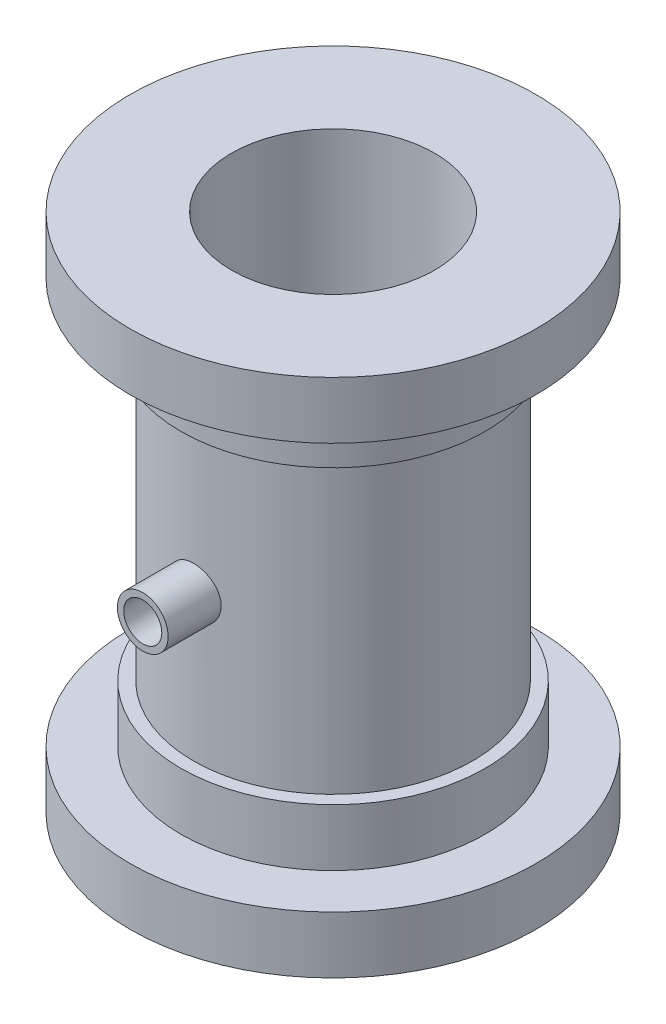
ISO-10303-21;
HEADER;
FILE_DESCRIPTION(('STEP AP214'),'2;1');
FILE_NAME('part.step','',(''),(''),'','','');
FILE_SCHEMA(('AUTOMOTIVE_DESIGN { 1 0 10303 214 1 1 1 1 }'));
ENDSEC;
DATA;
#1=APPLICATION_CONTEXT('core data for automotive mechanical design processes');
#2=APPLICATION_PROTOCOL_DEFINITION('international standard','automotive_design',2000,#1);
#3=PRODUCT_CONTEXT('',#1,'mechanical');
#4=PRODUCT('Part','Part','',(#3));
#5=PRODUCT_RELATED_PRODUCT_CATEGORY('part','',(#4));
#6=PRODUCT_DEFINITION_FORMATION('','',#4);
#7=PRODUCT_DEFINITION_CONTEXT('part definition',#1,'design');
#8=PRODUCT_DEFINITION('design','',#6,#7);
#9=PRODUCT_DEFINITION_SHAPE('','',#8);
#10=(LENGTH_UNIT() NAMED_UNIT(*) SI_UNIT(.MILLI.,.METRE.));
#11=(NAMED_UNIT(*) PLANE_ANGLE_UNIT() SI_UNIT($,.RADIAN.));
#12=(NAMED_UNIT(*) SI_UNIT($,.STERADIAN.) SOLID_ANGLE_UNIT());
#13=UNCERTAINTY_MEASURE_WITH_UNIT(LENGTH_MEASURE(1.E-05),#10,'distance_accuracy_value','');
#14=(GEOMETRIC_REPRESENTATION_CONTEXT(3) GLOBAL_UNCERTAINTY_ASSIGNED_CONTEXT((#13)) GLOBAL_UNIT_ASSIGNED_CONTEXT((#10,
#11,#12)) REPRESENTATION_CONTEXT('',''));
#15=CARTESIAN_POINT('',(0.,0.,0.));
#16=DIRECTION('',(0.,0.,1.));
#17=DIRECTION('',(1.,0.,0.));
#18=AXIS2_PLACEMENT_3D('',#15,#16,#17);
#19=CARTESIAN_POINT('',(0.,206.829787614374,0.));
#20=DIRECTION('',(0.,1.,0.));
#21=DIRECTION('',(0.,0.,1.));
#22=AXIS2_PLACEMENT_3D('',#19,#20,#21);
#23=CYLINDRICAL_SURFACE('',#22,16.);
#24=CARTESIAN_POINT('',(2.99999999999999,41.,-15.7162336455017));
#25=CARTESIAN_POINT('',(2.99999359766588,40.8330855839748,-15.7162368759014));
#26=CARTESIAN_POINT('',(2.98602252697897,40.6660881035627,-15.7189215952138));
#27=CARTESIAN_POINT('',(2.93054506503583,40.3368020768367,-15.7293570202788));
#28=CARTESIAN_POINT('',(2.88901531536946,40.1745176471452,-15.7371120234618));
#29=CARTESIAN_POINT('',(2.77974071235581,39.8594698572581,-15.7567795292999));
#30=CARTESIAN_POINT('',(2.71202027908749,39.7066977813854,-15.7686881581205));
#31=CARTESIAN_POINT('',(2.55235131520729,39.4146928814264,-15.7953165264186));
#32=CARTESIAN_POINT('',(2.46040467518385,39.2754590019934,-15.8100360465123));
#33=CARTESIAN_POINT('',(2.25367357885245,39.0127396016017,-15.840832296779));
#34=CARTESIAN_POINT('',(2.13864585866183,38.8894470330565,-15.8569223325136));
#35=CARTESIAN_POINT('',(1.8895435576071,38.6637912208009,-15.8885291532806));
#36=CARTESIAN_POINT('',(1.75546772724988,38.5614293511504,-15.904045900623));
#37=CARTESIAN_POINT('',(1.47080778914032,38.379801246799,-15.9329003565681));
#38=CARTESIAN_POINT('',(1.32010568006772,38.3007169329612,-15.9462205610472));
#39=CARTESIAN_POINT('',(1.00726256650152,38.1690609154529,-15.9690321726586));
#40=CARTESIAN_POINT('',(0.845122503719006,38.1164870320196,-15.9785238945667));
#41=CARTESIAN_POINT('',(0.516005492374828,38.0399409027777,-15.9925151024756));
#42=CARTESIAN_POINT('',(0.349106646489711,38.0156433881546,-15.9970713195265));
#43=CARTESIAN_POINT('',(0.0135433520707638,37.9953262245992,-16.0008736923119));
#44=CARTESIAN_POINT('',(-0.155120944895342,37.9993041677219,-16.0001203002139));
#45=CARTESIAN_POINT('',(-0.487196715798794,38.0351755422943,-15.9934326752648));
#46=CARTESIAN_POINT('',(-0.650647520902939,38.06671873886,-15.9875634449443));
#47=CARTESIAN_POINT('',(-0.969894331430951,38.1562712987905,-15.9713765266712));
#48=CARTESIAN_POINT('',(-1.12569005765308,38.2142816266916,-15.9610586765993));
#49=CARTESIAN_POINT('',(-1.42622013150304,38.3554554621166,-15.9370252059468));
#50=CARTESIAN_POINT('',(-1.57088714367706,38.438758975825,-15.9232907518165));
#51=CARTESIAN_POINT('',(-1.84431995442927,38.6280513381543,-15.893942950857));
#52=CARTESIAN_POINT('',(-1.97308413382157,38.7340424937752,-15.8783294130233));
#53=CARTESIAN_POINT('',(-2.21313123793807,38.9676314059671,-15.8466702736113));
#54=CARTESIAN_POINT('',(-2.32411581514081,39.0955355678042,-15.8306217180324));
#55=CARTESIAN_POINT('',(-2.5231034370252,39.3682990625573,-15.8001301784924));
#56=CARTESIAN_POINT('',(-2.61110614542363,39.5131586435293,-15.785687218027));
#57=CARTESIAN_POINT('',(-2.76171704448954,39.8161165414053,-15.7600378661424));
#58=CARTESIAN_POINT('',(-2.82428187290842,39.9742369143813,-15.7488370106052));
#59=CARTESIAN_POINT('',(-2.92187313950111,40.2990023682464,-15.7310248479338));
#60=CARTESIAN_POINT('',(-2.95690269802215,40.4656464809296,-15.7244130207724));
#61=CARTESIAN_POINT('',(-2.99799345299477,40.8000386577118,-15.7166304060201));
#62=CARTESIAN_POINT('',(-3.00448328571716,40.967732231131,-15.7153791163227));
#63=CARTESIAN_POINT('',(-2.98945937763448,41.3018069101743,-15.7182438284168));
#64=CARTESIAN_POINT('',(-2.96794702172865,41.4681880802962,-15.7223595647722));
#65=CARTESIAN_POINT('',(-2.89789736391764,41.7935058061088,-15.7354196012641));
#66=CARTESIAN_POINT('',(-2.84958477167978,41.9524925052498,-15.7443237338176));
#67=CARTESIAN_POINT('',(-2.72754448758118,42.2601143794603,-15.7659226831324));
#68=CARTESIAN_POINT('',(-2.65381492257589,42.4087487906307,-15.7786177792656));
#69=CARTESIAN_POINT('',(-2.48204706239319,42.6933352380863,-15.8065515572737));
#70=CARTESIAN_POINT('',(-2.38373799279241,42.8291210757322,-15.8218179085063));
#71=CARTESIAN_POINT('',(-2.16596688688492,43.0824240804287,-15.853096227362));
#72=CARTESIAN_POINT('',(-2.04650294866166,43.1999396031115,-15.8691082619299));
#73=CARTESIAN_POINT('',(-1.78789883574076,43.4149675270682,-15.9003324801189));
#74=CARTESIAN_POINT('',(-1.64851706819177,43.5121916532119,-15.9155311166661));
#75=CARTESIAN_POINT('',(-1.35514904608027,43.6818424123553,-15.943188096207));
#76=CARTESIAN_POINT('',(-1.20116335407705,43.75427000005,-15.9556465446945));
#77=CARTESIAN_POINT('',(-0.883755083157361,43.8718401957282,-15.9763611599169));
#78=CARTESIAN_POINT('',(-0.72038642615797,43.9171243751228,-15.9846390946028));
#79=CARTESIAN_POINT('',(-0.388192454763134,43.9795740965798,-15.9961528416749));
#80=CARTESIAN_POINT('',(-0.219367716431691,43.9967425973254,-15.9993891845988));
#81=CARTESIAN_POINT('',(0.116181520501017,44.0023706030369,-16.0004445503086));
#82=CARTESIAN_POINT('',(0.282898614132518,43.9912655062591,-15.9983457325));
#83=CARTESIAN_POINT('',(0.612046738558423,43.9416151444631,-15.9891373322347));
#84=CARTESIAN_POINT('',(0.774477810427464,43.9030701425114,-15.9820277978157));
#85=CARTESIAN_POINT('',(1.09021295119089,43.7998175852327,-15.9635967595586));
#86=CARTESIAN_POINT('',(1.24353263863614,43.7351563742386,-15.9522827196228));
#87=CARTESIAN_POINT('',(1.5372112626337,43.581559092689,-15.9266674413841));
#88=CARTESIAN_POINT('',(1.67756933000769,43.4926213957845,-15.912366002962));
#89=CARTESIAN_POINT('',(1.94351005555884,43.2914970911175,-15.882095597166));
#90=CARTESIAN_POINT('',(2.06885247077666,43.1789959322848,-15.8661056917023));
#91=CARTESIAN_POINT('',(2.29903072131409,42.9345908750064,-15.8343926708998));
#92=CARTESIAN_POINT('',(2.403861726512,42.8026824192219,-15.8186696191953));
#93=CARTESIAN_POINT('',(2.59095267889405,42.5217470906199,-15.7891115480538));
#94=CARTESIAN_POINT('',(2.67299481058046,42.3725731207714,-15.7752953438736));
#95=CARTESIAN_POINT('',(2.8107226484115,42.0623484201479,-15.7513416912985));
#96=CARTESIAN_POINT('',(2.86643323276462,41.9013090668493,-15.7412007725928));
#97=CARTESIAN_POINT('',(2.93859453193229,41.6164954238523,-15.7278603261271));
#98=CARTESIAN_POINT('',(2.96158211479938,41.4943885524718,-15.7235262144357));
#99=CARTESIAN_POINT('',(2.99228702152191,41.2482030631637,-15.7177117118331));
#100=CARTESIAN_POINT('',(3.00000476104181,41.1241244990007,-15.7162312432422));
#101=CARTESIAN_POINT('',(2.99999999999999,41.,-15.7162336455017));
#102=B_SPLINE_CURVE_WITH_KNOTS('',3,(#24,#25,#26,#27,#28,#29,#30,#31,#32,#33,#34,#35,#36,#37,
#38,#39,#40,#41,#42,#43,#44,#45,#46,#47,#48,#49,#50,#51,#52,#53,#54,#55,#56,#57,#58,#59,#60,#61,
#62,#63,#64,#65,#66,#67,#68,#69,#70,#71,#72,#73,#74,#75,#76,#77,#78,#79,#80,#81,#82,#83,#84,#85,
#86,#87,#88,#89,#90,#91,#92,#93,#94,#95,#96,#97,#98,#99,#100,#101),.UNSPECIFIED.,.T.,.F.,(4,2,2,
2,2,2,2,2,2,2,2,2,2,2,2,2,2,2,2,2,2,2,2,2,2,2,2,2,2,2,2,2,2,2,2,2,2,2,4),(0.,0.500289011586363,
1.00100260476078,1.50125045595686,2.00145927987815,2.50724671397381,3.01306734138628,
3.52274208696094,4.03237491879279,4.53608550920521,5.03975320401295,5.53711301197448,
6.03449094656847,6.53467383968437,7.03490761823569,7.54281229528126,8.05072440384797,
8.5594987223653,9.06821537732973,9.56926497174148,10.0702897867743,10.5671758463073,
11.0640985324863,11.5667572530828,12.0694611878935,12.5788825099174,13.0882842164341,
13.5950053883736,14.1016732333466,14.6005860114027,15.0994940064433,15.5975205306071,
16.0955804271421,16.6007692801748,17.1060769546152,17.6160600363781,18.1255603150175,
18.4976061505794,18.8696418584436),.UNSPECIFIED.);
#103=CARTESIAN_POINT('',(2.99999999999999,41.,-15.7162336455017));
#104=VERTEX_POINT('',#103);
#105=EDGE_CURVE('E41',#104,#104,#102,.T.);
#106=ORIENTED_EDGE('',*,*,#105,.T.);
#107=EDGE_LOOP('',(#106));
#108=FACE_BOUND('',#107,.T.);
#109=CARTESIAN_POINT('',(0.,0.,0.));
#110=DIRECTION('',(0.,1.,0.));
#111=DIRECTION('',(0.,0.,1.));
#112=AXIS2_PLACEMENT_3D('',#109,#110,#111);
#113=CIRCLE('',#112,16.);
#114=CARTESIAN_POINT('',(0.,0.,16.));
#115=VERTEX_POINT('',#114);
#116=EDGE_CURVE('E52',#115,#115,#113,.T.);
#117=ORIENTED_EDGE('',*,*,#116,.F.);
#118=EDGE_LOOP('',(#117));
#119=FACE_BOUND('',#118,.T.);
#120=CARTESIAN_POINT('',(0.,82.,0.));
#121=DIRECTION('',(0.,1.,0.));
#122=DIRECTION('',(0.,0.,1.));
#123=AXIS2_PLACEMENT_3D('',#120,#121,#122);
#124=CIRCLE('',#123,16.);
#125=CARTESIAN_POINT('',(0.,82.,16.));
#126=VERTEX_POINT('',#125);
#127=EDGE_CURVE('E47',#126,#126,#124,.T.);
#128=ORIENTED_EDGE('',*,*,#127,.T.);
#129=EDGE_LOOP('',(#128));
#130=FACE_BOUND('',#129,.T.);
#131=CARTESIAN_POINT('',(2.99999999999999,41.,15.7162336455017));
#132=CARTESIAN_POINT('',(2.99999359766588,40.8330855839748,15.7162368759014));
#133=CARTESIAN_POINT('',(2.98602252697897,40.6660881035627,15.7189215952138));
#134=CARTESIAN_POINT('',(2.93054506503583,40.3368020768367,15.7293570202788));
#135=CARTESIAN_POINT('',(2.88901531536946,40.1745176471452,15.7371120234618));
#136=CARTESIAN_POINT('',(2.77974071235581,39.8594698572581,15.7567795292999));
#137=CARTESIAN_POINT('',(2.71202027908749,39.7066977813854,15.7686881581205));
#138=CARTESIAN_POINT('',(2.55235131520729,39.4146928814264,15.7953165264186));
#139=CARTESIAN_POINT('',(2.46040467518385,39.2754590019934,15.8100360465123));
#140=CARTESIAN_POINT('',(2.25367357885245,39.0127396016017,15.840832296779));
#141=CARTESIAN_POINT('',(2.13864585866183,38.8894470330565,15.8569223325136));
#142=CARTESIAN_POINT('',(1.8895435576071,38.6637912208009,15.8885291532806));
#143=CARTESIAN_POINT('',(1.75546772724988,38.5614293511504,15.904045900623));
#144=CARTESIAN_POINT('',(1.47080778914032,38.379801246799,15.9329003565681));
#145=CARTESIAN_POINT('',(1.32010568006772,38.3007169329612,15.9462205610472));
#146=CARTESIAN_POINT('',(1.00726256650152,38.1690609154529,15.9690321726586));
#147=CARTESIAN_POINT('',(0.845122503719006,38.1164870320196,15.9785238945667));
#148=CARTESIAN_POINT('',(0.516005492374828,38.0399409027777,15.9925151024756));
#149=CARTESIAN_POINT('',(0.349106646489711,38.0156433881546,15.9970713195265));
#150=CARTESIAN_POINT('',(0.0135433520707638,37.9953262245992,16.0008736923119));
#151=CARTESIAN_POINT('',(-0.155120944895342,37.9993041677219,16.0001203002139));
#152=CARTESIAN_POINT('',(-0.487196715798794,38.0351755422943,15.9934326752648));
#153=CARTESIAN_POINT('',(-0.650647520902939,38.06671873886,15.9875634449443));
#154=CARTESIAN_POINT('',(-0.969894331430951,38.1562712987905,15.9713765266712));
#155=CARTESIAN_POINT('',(-1.12569005765308,38.2142816266916,15.9610586765993));
#156=CARTESIAN_POINT('',(-1.42622013150304,38.3554554621166,15.9370252059468));
#157=CARTESIAN_POINT('',(-1.57088714367706,38.438758975825,15.9232907518165));
#158=CARTESIAN_POINT('',(-1.84431995442927,38.6280513381543,15.893942950857));
#159=CARTESIAN_POINT('',(-1.97308413382157,38.7340424937752,15.8783294130233));
#160=CARTESIAN_POINT('',(-2.21313123793807,38.9676314059671,15.8466702736113));
#161=CARTESIAN_POINT('',(-2.32411581514081,39.0955355678042,15.8306217180324));
#162=CARTESIAN_POINT('',(-2.5231034370252,39.3682990625573,15.8001301784924));
#163=CARTESIAN_POINT('',(-2.61110614542363,39.5131586435293,15.785687218027));
#164=CARTESIAN_POINT('',(-2.76171704448954,39.8161165414053,15.7600378661424));
#165=CARTESIAN_POINT('',(-2.82428187290842,39.9742369143813,15.7488370106052));
#166=CARTESIAN_POINT('',(-2.92187313950111,40.2990023682464,15.7310248479338));
#167=CARTESIAN_POINT('',(-2.95690269802215,40.4656464809296,15.7244130207724));
#168=CARTESIAN_POINT('',(-2.99799345299477,40.8000386577118,15.7166304060201));
#169=CARTESIAN_POINT('',(-3.00448328571716,40.967732231131,15.7153791163227));
#170=CARTESIAN_POINT('',(-2.98945937763448,41.3018069101743,15.7182438284168));
#171=CARTESIAN_POINT('',(-2.96794702172865,41.4681880802962,15.7223595647722));
#172=CARTESIAN_POINT('',(-2.89789736391764,41.7935058061088,15.7354196012641));
#173=CARTESIAN_POINT('',(-2.84958477167978,41.9524925052498,15.7443237338176));
#174=CARTESIAN_POINT('',(-2.72754448758118,42.2601143794603,15.7659226831324));
#175=CARTESIAN_POINT('',(-2.65381492257589,42.4087487906307,15.7786177792656));
#176=CARTESIAN_POINT('',(-2.48204706239319,42.6933352380863,15.8065515572737));
#177=CARTESIAN_POINT('',(-2.38373799279241,42.8291210757322,15.8218179085063));
#178=CARTESIAN_POINT('',(-2.16596688688492,43.0824240804287,15.853096227362));
#179=CARTESIAN_POINT('',(-2.04650294866166,43.1999396031115,15.8691082619299));
#180=CARTESIAN_POINT('',(-1.78789883574076,43.4149675270682,15.9003324801189));
#181=CARTESIAN_POINT('',(-1.64851706819177,43.5121916532119,15.9155311166661));
#182=CARTESIAN_POINT('',(-1.35514904608027,43.6818424123553,15.943188096207));
#183=CARTESIAN_POINT('',(-1.20116335407705,43.75427000005,15.9556465446945));
#184=CARTESIAN_POINT('',(-0.883755083157361,43.8718401957282,15.9763611599169));
#185=CARTESIAN_POINT('',(-0.72038642615797,43.9171243751228,15.9846390946028));
#186=CARTESIAN_POINT('',(-0.388192454763134,43.9795740965798,15.9961528416749));
#187=CARTESIAN_POINT('',(-0.219367716431691,43.9967425973254,15.9993891845988));
#188=CARTESIAN_POINT('',(0.116181520501017,44.0023706030369,16.0004445503086));
#189=CARTESIAN_POINT('',(0.282898614132518,43.9912655062591,15.9983457325));
#190=CARTESIAN_POINT('',(0.612046738558423,43.9416151444631,15.9891373322347));
#191=CARTESIAN_POINT('',(0.774477810427464,43.9030701425114,15.9820277978157));
#192=CARTESIAN_POINT('',(1.09021295119089,43.7998175852327,15.9635967595586));
#193=CARTESIAN_POINT('',(1.24353263863614,43.7351563742386,15.9522827196228));
#194=CARTESIAN_POINT('',(1.5372112626337,43.581559092689,15.9266674413841));
#195=CARTESIAN_POINT('',(1.67756933000769,43.4926213957845,15.912366002962));
#196=CARTESIAN_POINT('',(1.94351005555884,43.2914970911175,15.882095597166));
#197=CARTESIAN_POINT('',(2.06885247077666,43.1789959322848,15.8661056917023));
#198=CARTESIAN_POINT('',(2.29903072131409,42.9345908750064,15.8343926708998));
#199=CARTESIAN_POINT('',(2.403861726512,42.8026824192219,15.8186696191953));
#200=CARTESIAN_POINT('',(2.59095267889405,42.5217470906199,15.7891115480538));
#201=CARTESIAN_POINT('',(2.67299481058046,42.3725731207714,15.7752953438736));
#202=CARTESIAN_POINT('',(2.8107226484115,42.0623484201479,15.7513416912985));
#203=CARTESIAN_POINT('',(2.86643323276462,41.9013090668493,15.7412007725928));
#204=CARTESIAN_POINT('',(2.93859453193229,41.6164954238523,15.7278603261271));
#205=CARTESIAN_POINT('',(2.96158211479938,41.4943885524718,15.7235262144357));
#206=CARTESIAN_POINT('',(2.99228702152191,41.2482030631637,15.7177117118331));
#207=CARTESIAN_POINT('',(3.00000476104181,41.1241244990007,15.7162312432422));
#208=CARTESIAN_POINT('',(2.99999999999999,41.,15.7162336455017));
#209=B_SPLINE_CURVE_WITH_KNOTS('',3,(#131,#132,#133,#134,#135,#136,#137,#138,#139,#140,#141,
#142,#143,#144,#145,#146,#147,#148,#149,#150,#151,#152,#153,#154,#155,#156,#157,#158,#159,#160,
#161,#162,#163,#164,#165,#166,#167,#168,#169,#170,#171,#172,#173,#174,#175,#176,#177,#178,#179,
#180,#181,#182,#183,#184,#185,#186,#187,#188,#189,#190,#191,#192,#193,#194,#195,#196,#197,#198,
#199,#200,#201,#202,#203,#204,#205,#206,#207,#208),.UNSPECIFIED.,.T.,.F.,(4,2,2,2,2,2,2,2,2,2,2,
2,2,2,2,2,2,2,2,2,2,2,2,2,2,2,2,2,2,2,2,2,2,2,2,2,2,2,4),(0.,0.500289011586363,1.00100260476078,
1.50125045595686,2.00145927987815,2.50724671397381,3.01306734138628,3.52274208696094,
4.03237491879279,4.53608550920521,5.03975320401295,5.53711301197448,6.03449094656847,
6.53467383968437,7.03490761823569,7.54281229528126,8.05072440384797,8.5594987223653,
9.06821537732973,9.56926497174148,10.0702897867743,10.5671758463073,11.0640985324863,
11.5667572530828,12.0694611878935,12.5788825099174,13.0882842164341,13.5950053883736,
14.1016732333466,14.6005860114027,15.0994940064433,15.5975205306071,16.0955804271421,
16.6007692801748,17.1060769546152,17.6160600363781,18.1255603150175,18.4976061505794,
18.8696418584436),.UNSPECIFIED.);
#210=CARTESIAN_POINT('',(2.99999999999999,41.,15.7162336455017));
#211=VERTEX_POINT('',#210);
#212=EDGE_CURVE('E149',#211,#211,#209,.T.);
#213=ORIENTED_EDGE('',*,*,#212,.F.);
#214=EDGE_LOOP('',(#213));
#215=FACE_BOUND('',#214,.T.);
#216=ADVANCED_FACE('F40',(#108,#119,#130,#215),#23,.F.);
#217=CARTESIAN_POINT('',(0.,206.829787614374,0.));
#218=DIRECTION('',(0.,1.,0.));
#219=DIRECTION('',(0.,0.,1.));
#220=AXIS2_PLACEMENT_3D('',#217,#218,#219);
#221=CYLINDRICAL_SURFACE('',#220,22.);
#222=CARTESIAN_POINT('',(2.99999999999999,41.,-21.7944947177034));
#223=CARTESIAN_POINT('',(2.99999295397828,41.1676686557939,-21.7944973125222));
#224=CARTESIAN_POINT('',(2.98589613516891,41.335438885572,-21.7964504822141));
#225=CARTESIAN_POINT('',(2.92988930626151,41.6663009494034,-21.8040481680046));
#226=CARTESIAN_POINT('',(2.88795106929476,41.8293878600565,-21.8096964302678));
#227=CARTESIAN_POINT('',(2.7775288562679,42.1460455710164,-21.8240329226108));
#228=CARTESIAN_POINT('',(2.70906391400625,42.2996231031868,-21.8327189725423));
#229=CARTESIAN_POINT('',(2.54757436301585,42.593083937498,-21.8521497354893));
#230=CARTESIAN_POINT('',(2.4545535979434,42.7329693781315,-21.8628941262462));
#231=CARTESIAN_POINT('',(2.24593261550095,42.9960291899694,-21.8853107439761));
#232=CARTESIAN_POINT('',(2.13020174404837,43.1190995206715,-21.8969880962733));
#233=CARTESIAN_POINT('',(1.87972745186893,43.3441356113716,-21.9199089625179));
#234=CARTESIAN_POINT('',(1.74498304377951,43.446100274685,-21.9311524538967));
#235=CARTESIAN_POINT('',(1.45964673364284,43.6264088097933,-21.9519917823356));
#236=CARTESIAN_POINT('',(1.30899431491146,43.7046577531438,-21.9615809332171));
#237=CARTESIAN_POINT('',(0.996533559622191,43.8347051362175,-21.9779746087792));
#238=CARTESIAN_POINT('',(0.834725713012592,43.8865047367613,-21.9847792556648));
#239=CARTESIAN_POINT('',(0.505615027627403,43.9618700639319,-21.9948010960819));
#240=CARTESIAN_POINT('',(0.338352625202418,43.9856093917029,-21.9980403391051));
#241=CARTESIAN_POINT('',(0.00218901989865064,44.0047187619281,-22.0006418160325));
#242=CARTESIAN_POINT('',(-0.166712106612742,44.0000901200993,-22.0000042297454));
#243=CARTESIAN_POINT('',(-0.500176134095491,43.9627331448272,-21.9949416293269));
#244=CARTESIAN_POINT('',(-0.664760389901238,43.9301915409683,-21.9905417842193));
#245=CARTESIAN_POINT('',(-0.986109968659578,43.8382247979685,-21.9784771616625));
#246=CARTESIAN_POINT('',(-1.1428751195119,43.7787990673916,-21.9708123123852));
#247=CARTESIAN_POINT('',(-1.44470900216683,43.6345555950203,-21.9530355245634));
#248=CARTESIAN_POINT('',(-1.58973910165001,43.5496579984127,-21.9429159096715));
#249=CARTESIAN_POINT('',(-1.86356465940336,43.356938901094,-21.9213599095811));
#250=CARTESIAN_POINT('',(-1.99235923191068,43.2491161505149,-21.9099234526045));
#251=CARTESIAN_POINT('',(-2.2311563912285,43.0125639881593,-21.8869019715346));
#252=CARTESIAN_POINT('',(-2.34099765683571,42.883671704982,-21.8753164955576));
#253=CARTESIAN_POINT('',(-2.53751386076588,42.6091960813263,-21.8533940433535));
#254=CARTESIAN_POINT('',(-2.62418869928228,42.4636126689425,-21.8430570725053));
#255=CARTESIAN_POINT('',(-2.77192629130126,42.159733098398,-21.8248023099056));
#256=CARTESIAN_POINT('',(-2.83297454471216,42.0014298032314,-21.816885888441));
#257=CARTESIAN_POINT('',(-2.92757469616753,41.6766859388551,-21.8043941534575));
#258=CARTESIAN_POINT('',(-2.96112818173422,41.5102458400451,-21.7998186470391));
#259=CARTESIAN_POINT('',(-2.99956941672118,41.1753823129862,-21.7945626889125));
#260=CARTESIAN_POINT('',(-3.00468490854896,41.006985496761,-21.7938512929769));
#261=CARTESIAN_POINT('',(-2.98670732293098,40.6717371641337,-21.7963221316711));
#262=CARTESIAN_POINT('',(-2.96361496443093,40.5048856084559,-21.7995042670648));
#263=CARTESIAN_POINT('',(-2.89006955453773,40.1781565348422,-21.8093753071634));
#264=CARTESIAN_POINT('',(-2.83972815512374,40.0182534145076,-21.8160498979624));
#265=CARTESIAN_POINT('',(-2.71322912313732,39.7091565507405,-21.8321421092609));
#266=CARTESIAN_POINT('',(-2.63707042220061,39.5599632508084,-21.8415598432741));
#267=CARTESIAN_POINT('',(-2.46054424209314,39.2754947875546,-21.8621508077798));
#268=CARTESIAN_POINT('',(-2.36002824545062,39.1403125677473,-21.8733346554527));
#269=CARTESIAN_POINT('',(-2.13784918546697,38.8886549951314,-21.8961649833416));
#270=CARTESIAN_POINT('',(-2.01618513932771,38.7721805121983,-21.9078114850387));
#271=CARTESIAN_POINT('',(-1.7541651749027,38.5604369463813,-21.9303506440045));
#272=CARTESIAN_POINT('',(-1.61368731048534,38.4653180710751,-21.9412376115705));
#273=CARTESIAN_POINT('',(-1.31861563564172,38.3000282219224,-21.9609445601932));
#274=CARTESIAN_POINT('',(-1.16402215510119,38.229856665238,-21.9697645895377));
#275=CARTESIAN_POINT('',(-0.845593617063874,38.116697948143,-21.9843187797623));
#276=CARTESIAN_POINT('',(-0.681789143548591,38.0736260127072,-21.9900625555325));
#277=CARTESIAN_POINT('',(-0.349189125620999,38.0156139846478,-21.9978571930975));
#278=CARTESIAN_POINT('',(-0.18039385182202,38.0006723695607,-21.9999082547485));
#279=CARTESIAN_POINT('',(0.155933944793781,37.9993773344575,-22.0000849669784));
#280=CARTESIAN_POINT('',(0.323465608546994,38.0127930862346,-21.9982423123403));
#281=CARTESIAN_POINT('',(0.65386852750444,38.0673405312772,-21.9909020074537));
#282=CARTESIAN_POINT('',(0.816739790572315,38.1084721777741,-21.9854043633727));
#283=CARTESIAN_POINT('',(1.13315387765858,38.2172071855912,-21.9713688879314));
#284=CARTESIAN_POINT('',(1.28670131426866,38.2847973323295,-21.9628325744139));
#285=CARTESIAN_POINT('',(1.58031159285156,38.4445066044813,-21.9436616719154));
#286=CARTESIAN_POINT('',(1.72037415250691,38.5366262432889,-21.9330270390184));
#287=CARTESIAN_POINT('',(1.98421472860386,38.7436255734436,-21.9107413064255));
#288=CARTESIAN_POINT('',(2.10785776937318,38.8586765359164,-21.899082951343));
#289=CARTESIAN_POINT('',(2.33416948478684,39.1079137559864,-21.8761200052605));
#290=CARTESIAN_POINT('',(2.43683320845294,39.2421045177904,-21.864815498298));
#291=CARTESIAN_POINT('',(2.61868613380123,39.5265296933573,-21.8437846234674));
#292=CARTESIAN_POINT('',(2.69776514213642,39.6768350915978,-21.8340657568726));
#293=CARTESIAN_POINT('',(2.82944291998179,39.9886475846397,-21.817394367016));
#294=CARTESIAN_POINT('',(2.8820699216208,40.1501425264417,-21.8104388960614));
#295=CARTESIAN_POINT('',(2.94703203226376,40.427022796486,-21.8017355288375));
#296=CARTESIAN_POINT('',(2.96686567785598,40.5406764223968,-21.7990341203125));
#297=CARTESIAN_POINT('',(2.99335201931174,40.7695373771214,-21.7954128315745));
#298=CARTESIAN_POINT('',(3.00000484343007,40.8847446908062,-21.7944929340268));
#299=CARTESIAN_POINT('',(2.99999999999999,41.,-21.7944947177034));
#300=B_SPLINE_CURVE_WITH_KNOTS('',3,(#222,#223,#224,#225,#226,#227,#228,#229,#230,#231,#232,
#233,#234,#235,#236,#237,#238,#239,#240,#241,#242,#243,#244,#245,#246,#247,#248,#249,#250,#251,
#252,#253,#254,#255,#256,#257,#258,#259,#260,#261,#262,#263,#264,#265,#266,#267,#268,#269,#270,
#271,#272,#273,#274,#275,#276,#277,#278,#279,#280,#281,#282,#283,#284,#285,#286,#287,#288,#289,
#290,#291,#292,#293,#294,#295,#296,#297,#298,#299),.UNSPECIFIED.,.T.,.F.,(4,2,2,2,2,2,2,2,2,2,2,
2,2,2,2,2,2,2,2,2,2,2,2,2,2,2,2,2,2,2,2,2,2,2,2,2,2,2,4),(0.,0.502584827322537,1.00567997726411,
1.50841480614355,2.01107098991681,2.51670860353079,3.02237248429927,3.53003447052539,
4.03767417433727,4.54215653413512,5.04661549603349,5.54772586150295,6.04884725166252,
6.55155638132179,7.05429292546102,7.56111742626898,8.06794411056384,8.57505718337531,
9.0821409738876,9.585157927571,10.0881620609109,10.5891205844915,11.0900998411272,
11.5942142584275,12.0983521093422,12.6059319233779,13.1134998781726,13.6194720220333,
14.125416780985,14.627259029653,15.1291004314968,15.6306915099823,16.1322930874247,
16.6377918045004,17.143409678468,17.6513541852325,18.158755407386,18.5042352052811,
18.8497116414994),.UNSPECIFIED.);
#301=CARTESIAN_POINT('',(2.99999999999999,41.,-21.7944947177034));
#302=VERTEX_POINT('',#301);
#303=EDGE_CURVE('E165',#302,#302,#300,.T.);
#304=ORIENTED_EDGE('',*,*,#303,.T.);
#305=EDGE_LOOP('',(#304));
#306=FACE_BOUND('',#305,.T.);
#307=CARTESIAN_POINT('',(0.,64.,0.));
#308=DIRECTION('',(0.,1.,0.));
#309=DIRECTION('',(0.,0.,1.));
#310=AXIS2_PLACEMENT_3D('',#307,#308,#309);
#311=CIRCLE('',#310,22.);
#312=CARTESIAN_POINT('',(0.,64.,22.));
#313=VERTEX_POINT('',#312);
#314=EDGE_CURVE('E184',#313,#313,#311,.T.);
#315=ORIENTED_EDGE('',*,*,#314,.F.);
#316=EDGE_LOOP('',(#315));
#317=FACE_BOUND('',#316,.T.);
#318=CARTESIAN_POINT('',(0.,18.,0.));
#319=DIRECTION('',(0.,1.,0.));
#320=DIRECTION('',(0.,0.,1.));
#321=AXIS2_PLACEMENT_3D('',#318,#319,#320);
#322=CIRCLE('',#321,22.);
#323=CARTESIAN_POINT('',(0.,18.,22.));
#324=VERTEX_POINT('',#323);
#325=EDGE_CURVE('E131',#324,#324,#322,.T.);
#326=ORIENTED_EDGE('',*,*,#325,.T.);
#327=EDGE_LOOP('',(#326));
#328=FACE_BOUND('',#327,.T.);
#329=CARTESIAN_POINT('',(0.,37.,22.));
#330=CARTESIAN_POINT('',(0.222714543288747,37.0000086373214,21.9999960145572));
#331=CARTESIAN_POINT('',(0.445542899836406,37.0186635149653,21.9965830546687));
#332=CARTESIAN_POINT('',(0.884928813696619,37.0927469320498,21.9832969500399));
#333=CARTESIAN_POINT('',(1.10148077453215,37.1482072971627,21.9734182144508));
#334=CARTESIAN_POINT('',(1.5218951450275,37.294154259342,21.9483064647013));
#335=CARTESIAN_POINT('',(1.72576852786036,37.3846100643795,21.9330781586384));
#336=CARTESIAN_POINT('',(2.11542400676901,37.5978946623836,21.898933429966));
#337=CARTESIAN_POINT('',(2.30120773535809,37.7207205303764,21.8800173406264));
#338=CARTESIAN_POINT('',(2.65152888102477,37.9967318192854,21.8403486699966));
#339=CARTESIAN_POINT('',(2.81583245206692,38.1502116839615,21.8195794519416));
#340=CARTESIAN_POINT('',(3.11650714682159,38.4825407081797,21.7786699042361));
#341=CARTESIAN_POINT('',(3.25287633589955,38.6613916233783,21.7585296182252));
#342=CARTESIAN_POINT('',(3.49477390032954,39.0410254589196,21.7209968041953));
#343=CARTESIAN_POINT('',(3.60006626531112,39.2419610704608,21.703625742202));
#344=CARTESIAN_POINT('',(3.77531093899957,39.6590373006479,21.673831665538));
#345=CARTESIAN_POINT('',(3.8452661056655,39.8751766880501,21.6614082507349));
#346=CARTESIAN_POINT('',(3.9471039542263,40.3140292987132,21.6430830703341));
#347=CARTESIAN_POINT('',(3.9793933285089,40.5366451834193,21.6371116924469));
#348=CARTESIAN_POINT('',(4.00624497473377,40.9842088146291,21.6321566286462));
#349=CARTESIAN_POINT('',(4.00081042593285,41.2091563630321,21.633172353881));
#350=CARTESIAN_POINT('',(3.95269868854,41.652063828266,21.6420133009836));
#351=CARTESIAN_POINT('',(3.91048235398145,41.8700757357914,21.6497542562853));
#352=CARTESIAN_POINT('',(3.79073046680053,42.2958700367343,21.6710412254782));
#353=CARTESIAN_POINT('',(3.71319349486377,42.5036520187036,21.6845874726463));
#354=CARTESIAN_POINT('',(3.52454595578591,42.9044455815575,21.7160476310543));
#355=CARTESIAN_POINT('',(3.4132478074308,43.0973668853323,21.733985834287));
#356=CARTESIAN_POINT('',(3.16037006748086,43.4619694738906,21.7721924402343));
#357=CARTESIAN_POINT('',(3.01878758047169,43.6336487252925,21.7924610656694));
#358=CARTESIAN_POINT('',(2.70686798836704,43.9535579928888,21.8334128161709));
#359=CARTESIAN_POINT('',(2.53613634531379,44.1014033768738,21.8540976363293));
#360=CARTESIAN_POINT('',(2.17208908138662,44.3664102669617,21.8932750087418));
#361=CARTESIAN_POINT('',(1.97877325899631,44.4835714992425,21.9117675414312));
#362=CARTESIAN_POINT('',(1.57465519699459,44.6839347795701,21.9445107565068));
#363=CARTESIAN_POINT('',(1.36383356079098,44.767098537392,21.9587566511844));
#364=CARTESIAN_POINT('',(0.930896828925329,44.8967263849874,21.9813641094176));
#365=CARTESIAN_POINT('',(0.708782862632127,44.9431941371478,21.9897262601819));
#366=CARTESIAN_POINT('',(0.262877299156996,44.9975795238382,21.9995438675732));
#367=CARTESIAN_POINT('',(0.0391520242178662,45.0060244469082,22.0010937868229));
#368=CARTESIAN_POINT('',(-0.406514477941937,44.985536403637,21.99737260495));
#369=CARTESIAN_POINT('',(-0.628455786906166,44.9566051598565,21.9921018181742));
#370=CARTESIAN_POINT('',(-1.06259419518552,44.8626245008763,21.975390172649));
#371=CARTESIAN_POINT('',(-1.27485059491664,44.7978402616343,21.9639946314432));
#372=CARTESIAN_POINT('',(-1.68548942751322,44.6342783429561,21.9363059024444));
#373=CARTESIAN_POINT('',(-1.8838709619219,44.5354984646046,21.9200123978487));
#374=CARTESIAN_POINT('',(-2.26339049414987,44.3055707243942,21.8840995916968));
#375=CARTESIAN_POINT('',(-2.44432890416976,44.1740986256881,21.864447632292));
#376=CARTESIAN_POINT('',(-2.78176427644695,43.8829592466578,21.8240857614217));
#377=CARTESIAN_POINT('',(-2.93825909948665,43.7232895011761,21.8033757575701));
#378=CARTESIAN_POINT('',(-3.2243547577536,43.377906237103,21.7629207911529));
#379=CARTESIAN_POINT('',(-3.35359673482837,43.1918933869483,21.7431910424377));
#380=CARTESIAN_POINT('',(-3.57899973104028,42.800487637187,21.7072302016204));
#381=CARTESIAN_POINT('',(-3.6751619326159,42.5950954306312,21.6909989844708));
#382=CARTESIAN_POINT('',(-3.83115890483493,42.1716985006165,21.6639908923095));
#383=CARTESIAN_POINT('',(-3.8911621572368,41.9537575385239,21.653188760335));
#384=CARTESIAN_POINT('',(-3.97366080357108,41.5106740227379,21.6382025309078));
#385=CARTESIAN_POINT('',(-3.99616014907258,41.2855322303022,21.6340177362272));
#386=CARTESIAN_POINT('',(-4.00288627326368,40.8380292490727,21.6327738776523));
#387=CARTESIAN_POINT('',(-3.98767874002465,40.6156766571229,21.6356094908823));
#388=CARTESIAN_POINT('',(-3.92065693825629,40.1767527239652,21.6478541749405));
#389=CARTESIAN_POINT('',(-3.86884285811435,39.9601813530114,21.6572632119402));
#390=CARTESIAN_POINT('',(-3.73031134316953,39.5392476052093,21.6815514416183));
#391=CARTESIAN_POINT('',(-3.64365162038465,39.3348656795531,21.6964215859949));
#392=CARTESIAN_POINT('',(-3.43794947329646,38.9434511056705,21.7299635502969));
#393=CARTESIAN_POINT('',(-3.31890495138014,38.7564195823088,21.7486356164588));
#394=CARTESIAN_POINT('',(-3.04983087325598,38.4021742508088,21.7880064930293));
#395=CARTESIAN_POINT('',(-2.89938831106199,38.2352768602585,21.8087301566221));
#396=CARTESIAN_POINT('',(-2.57265302846729,37.9289058379756,21.849679841373));
#397=CARTESIAN_POINT('',(-2.39635437360187,37.7894385192155,21.8699057470383));
#398=CARTESIAN_POINT('',(-2.0211423792926,37.540799405753,21.9077794859438));
#399=CARTESIAN_POINT('',(-1.82205169958099,37.4318916296397,21.9254042634686));
#400=CARTESIAN_POINT('',(-1.40814781017269,37.2492415678519,21.9558652198669));
#401=CARTESIAN_POINT('',(-1.19334985097334,37.1754656814434,21.9687059716947));
#402=CARTESIAN_POINT('',(-0.814883498916811,37.0804491393956,21.9854814075298));
#403=CARTESIAN_POINT('',(-0.653450854552979,37.0503313340793,21.9908956054717));
#404=CARTESIAN_POINT('',(-0.328032684264406,37.0101038124102,21.9981563286609));
#405=CARTESIAN_POINT('',(-0.164047216881666,36.9999936379165,22.0000029356));
#406=CARTESIAN_POINT('',(0.,37.,22.));
#407=B_SPLINE_CURVE_WITH_KNOTS('',3,(#329,#330,#331,#332,#333,#334,#335,#336,#337,#338,#339,
#340,#341,#342,#343,#344,#345,#346,#347,#348,#349,#350,#351,#352,#353,#354,#355,#356,#357,#358,
#359,#360,#361,#362,#363,#364,#365,#366,#367,#368,#369,#370,#371,#372,#373,#374,#375,#376,#377,
#378,#379,#380,#381,#382,#383,#384,#385,#386,#387,#388,#389,#390,#391,#392,#393,#394,#395,#396,
#397,#398,#399,#400,#401,#402,#403,#404,#405,#406),.UNSPECIFIED.,.T.,.F.,(4,2,2,2,2,2,2,2,2,2,2,
2,2,2,2,2,2,2,2,2,2,2,2,2,2,2,2,2,2,2,2,2,2,2,2,2,2,2,4),(0.,0.667543783104665,1.33566554414518,
2.00320076573349,2.67067568920301,3.34490029193771,4.01917157326157,4.69843904407301,
5.37765156911462,6.0494604234529,6.72121266048404,7.3846673458179,8.04814869357741,
8.71538612923251,9.38268738642511,10.0598642088374,10.7370470740929,11.4149905404762,
12.0928663372291,12.7613120199473,13.429726897016,14.0932628657086,14.7568417614844,
15.4272845359133,16.0977859523225,16.7766301226092,17.4554500250495,18.1310820215231,
18.806642826072,19.4721301946074,20.1376141383862,20.8020004051792,21.4664297155381,
22.1402222906008,22.8141697565893,23.4937720908586,24.1727231299633,24.6644342045912,
25.1561340197353),.UNSPECIFIED.);
#408=CARTESIAN_POINT('',(0.,37.,22.));
#409=VERTEX_POINT('',#408);
#410=EDGE_CURVE('E10',#409,#409,#407,.T.);
#411=ORIENTED_EDGE('',*,*,#410,.F.);
#412=EDGE_LOOP('',(#411));
#413=FACE_BOUND('',#412,.T.);
#414=ADVANCED_FACE('F62',(#306,#317,#328,#413),#221,.T.);
#415=CARTESIAN_POINT('',(32.,82.,0.));
#416=DIRECTION('',(0.,-1.,0.));
#417=DIRECTION('',(0.,0.,-1.));
#418=AXIS2_PLACEMENT_3D('',#415,#416,#417);
#419=PLANE('',#418);
#420=ORIENTED_EDGE('',*,*,#127,.F.);
#421=EDGE_LOOP('',(#420));
#422=FACE_BOUND('',#421,.T.);
#423=CARTESIAN_POINT('',(0.,82.,0.));
#424=DIRECTION('',(0.,1.,0.));
#425=DIRECTION('',(0.,0.,1.));
#426=AXIS2_PLACEMENT_3D('',#423,#424,#425);
#427=CIRCLE('',#426,32.);
#428=CARTESIAN_POINT('',(0.,82.,32.));
#429=VERTEX_POINT('',#428);
#430=EDGE_CURVE('E173',#429,#429,#427,.T.);
#431=ORIENTED_EDGE('',*,*,#430,.T.);
#432=EDGE_LOOP('',(#431));
#433=FACE_BOUND('',#432,.T.);
#434=ADVANCED_FACE('F39',(#422,#433),#419,.F.);
#435=CARTESIAN_POINT('',(16.,0.,0.));
#436=DIRECTION('',(0.,1.,0.));
#437=DIRECTION('',(0.,0.,1.));
#438=AXIS2_PLACEMENT_3D('',#435,#436,#437);
#439=PLANE('',#438);
#440=CARTESIAN_POINT('',(0.,0.,0.));
#441=DIRECTION('',(0.,1.,0.));
#442=DIRECTION('',(0.,0.,1.));
#443=AXIS2_PLACEMENT_3D('',#440,#441,#442);
#444=CIRCLE('',#443,32.);
#445=CARTESIAN_POINT('',(0.,0.,32.));
#446=VERTEX_POINT('',#445);
#447=EDGE_CURVE('E133',#446,#446,#444,.T.);
#448=ORIENTED_EDGE('',*,*,#447,.F.);
#449=EDGE_LOOP('',(#448));
#450=FACE_BOUND('',#449,.T.);
#451=ORIENTED_EDGE('',*,*,#116,.T.);
#452=EDGE_LOOP('',(#451));
#453=FACE_BOUND('',#452,.T.);
#454=ADVANCED_FACE('F110',(#450,#453),#439,.F.);
#455=CARTESIAN_POINT('',(0.,206.829787614374,0.));
#456=DIRECTION('',(0.,1.,0.));
#457=DIRECTION('',(0.,0.,1.));
#458=AXIS2_PLACEMENT_3D('',#455,#456,#457);
#459=CYLINDRICAL_SURFACE('',#458,32.);
#460=CARTESIAN_POINT('',(0.,9.00000000000001,0.));
#461=DIRECTION('',(0.,1.,0.));
#462=DIRECTION('',(0.,0.,1.));
#463=AXIS2_PLACEMENT_3D('',#460,#461,#462);
#464=CIRCLE('',#463,32.);
#465=CARTESIAN_POINT('',(0.,9.00000000000001,32.));
#466=VERTEX_POINT('',#465);
#467=EDGE_CURVE('E128',#466,#466,#464,.T.);
#468=ORIENTED_EDGE('',*,*,#467,.F.);
#469=EDGE_LOOP('',(#468));
#470=FACE_BOUND('',#469,.T.);
#471=ORIENTED_EDGE('',*,*,#447,.T.);
#472=EDGE_LOOP('',(#471));
#473=FACE_BOUND('',#472,.T.);
#474=ADVANCED_FACE('F109',(#470,#473),#459,.T.);
#475=CARTESIAN_POINT('',(32.,9.,0.));
#476=DIRECTION('',(0.,-1.,0.));
#477=DIRECTION('',(0.,0.,-1.));
#478=AXIS2_PLACEMENT_3D('',#475,#476,#477);
#479=PLANE('',#478);
#480=CARTESIAN_POINT('',(0.,9.00000000000001,0.));
#481=DIRECTION('',(0.,1.,0.));
#482=DIRECTION('',(0.,0.,1.));
#483=AXIS2_PLACEMENT_3D('',#480,#481,#482);
#484=CIRCLE('',#483,24.);
#485=CARTESIAN_POINT('',(0.,9.00000000000001,24.));
#486=VERTEX_POINT('',#485);
#487=EDGE_CURVE('E126',#486,#486,#484,.T.);
#488=ORIENTED_EDGE('',*,*,#487,.F.);
#489=EDGE_LOOP('',(#488));
#490=FACE_BOUND('',#489,.T.);
#491=ORIENTED_EDGE('',*,*,#467,.T.);
#492=EDGE_LOOP('',(#491));
#493=FACE_BOUND('',#492,.T.);
#494=ADVANCED_FACE('F112',(#490,#493),#479,.F.);
#495=CARTESIAN_POINT('',(0.,206.829787614374,0.));
#496=DIRECTION('',(0.,1.,0.));
#497=DIRECTION('',(0.,0.,1.));
#498=AXIS2_PLACEMENT_3D('',#495,#496,#497);
#499=CYLINDRICAL_SURFACE('',#498,24.);
#500=CARTESIAN_POINT('',(0.,18.,0.));
#501=DIRECTION('',(0.,1.,0.));
#502=DIRECTION('',(0.,0.,1.));
#503=AXIS2_PLACEMENT_3D('',#500,#501,#502);
#504=CIRCLE('',#503,24.);
#505=CARTESIAN_POINT('',(0.,18.,24.));
#506=VERTEX_POINT('',#505);
#507=EDGE_CURVE('E127',#506,#506,#504,.T.);
#508=ORIENTED_EDGE('',*,*,#507,.F.);
#509=EDGE_LOOP('',(#508));
#510=FACE_BOUND('',#509,.T.);
#511=ORIENTED_EDGE('',*,*,#487,.T.);
#512=EDGE_LOOP('',(#511));
#513=FACE_BOUND('',#512,.T.);
#514=ADVANCED_FACE('F93',(#510,#513),#499,.T.);
#515=CARTESIAN_POINT('',(24.,18.,0.));
#516=DIRECTION('',(0.,-1.,0.));
#517=DIRECTION('',(0.,0.,-1.));
#518=AXIS2_PLACEMENT_3D('',#515,#516,#517);
#519=PLANE('',#518);
#520=ORIENTED_EDGE('',*,*,#325,.F.);
#521=EDGE_LOOP('',(#520));
#522=FACE_BOUND('',#521,.T.);
#523=ORIENTED_EDGE('',*,*,#507,.T.);
#524=EDGE_LOOP('',(#523));
#525=FACE_BOUND('',#524,.T.);
#526=ADVANCED_FACE('F87',(#522,#525),#519,.F.);
#527=CARTESIAN_POINT('',(22.,64.,0.));
#528=DIRECTION('',(0.,1.,0.));
#529=DIRECTION('',(0.,0.,1.));
#530=AXIS2_PLACEMENT_3D('',#527,#528,#529);
#531=PLANE('',#530);
#532=CARTESIAN_POINT('',(0.,64.,0.));
#533=DIRECTION('',(0.,1.,0.));
#534=DIRECTION('',(0.,0.,1.));
#535=AXIS2_PLACEMENT_3D('',#532,#533,#534);
#536=CIRCLE('',#535,24.);
#537=CARTESIAN_POINT('',(0.,64.,24.));
#538=VERTEX_POINT('',#537);
#539=EDGE_CURVE('E185',#538,#538,#536,.T.);
#540=ORIENTED_EDGE('',*,*,#539,.F.);
#541=EDGE_LOOP('',(#540));
#542=FACE_BOUND('',#541,.T.);
#543=ORIENTED_EDGE('',*,*,#314,.T.);
#544=EDGE_LOOP('',(#543));
#545=FACE_BOUND('',#544,.T.);
#546=ADVANCED_FACE('F84',(#542,#545),#531,.F.);
#547=CARTESIAN_POINT('',(0.,206.829787614374,0.));
#548=DIRECTION('',(0.,1.,0.));
#549=DIRECTION('',(0.,0.,1.));
#550=AXIS2_PLACEMENT_3D('',#547,#548,#549);
#551=CYLINDRICAL_SURFACE('',#550,24.);
#552=CARTESIAN_POINT('',(0.,73.,0.));
#553=DIRECTION('',(0.,1.,0.));
#554=DIRECTION('',(0.,0.,1.));
#555=AXIS2_PLACEMENT_3D('',#552,#553,#554);
#556=CIRCLE('',#555,24.);
#557=CARTESIAN_POINT('',(0.,73.,24.));
#558=VERTEX_POINT('',#557);
#559=EDGE_CURVE('E177',#558,#558,#556,.T.);
#560=ORIENTED_EDGE('',*,*,#559,.F.);
#561=EDGE_LOOP('',(#560));
#562=FACE_BOUND('',#561,.T.);
#563=ORIENTED_EDGE('',*,*,#539,.T.);
#564=EDGE_LOOP('',(#563));
#565=FACE_BOUND('',#564,.T.);
#566=ADVANCED_FACE('F78',(#562,#565),#551,.T.);
#567=CARTESIAN_POINT('',(24.,73.,0.));
#568=DIRECTION('',(0.,1.,0.));
#569=DIRECTION('',(0.,0.,1.));
#570=AXIS2_PLACEMENT_3D('',#567,#568,#569);
#571=PLANE('',#570);
#572=CARTESIAN_POINT('',(0.,73.,0.));
#573=DIRECTION('',(0.,1.,0.));
#574=DIRECTION('',(0.,0.,1.));
#575=AXIS2_PLACEMENT_3D('',#572,#573,#574);
#576=CIRCLE('',#575,32.);
#577=CARTESIAN_POINT('',(0.,73.,32.));
#578=VERTEX_POINT('',#577);
#579=EDGE_CURVE('E176',#578,#578,#576,.T.);
#580=ORIENTED_EDGE('',*,*,#579,.F.);
#581=EDGE_LOOP('',(#580));
#582=FACE_BOUND('',#581,.T.);
#583=ORIENTED_EDGE('',*,*,#559,.T.);
#584=EDGE_LOOP('',(#583));
#585=FACE_BOUND('',#584,.T.);
#586=ADVANCED_FACE('F77',(#582,#585),#571,.F.);
#587=CARTESIAN_POINT('',(0.,206.829787614374,0.));
#588=DIRECTION('',(0.,1.,0.));
#589=DIRECTION('',(0.,0.,1.));
#590=AXIS2_PLACEMENT_3D('',#587,#588,#589);
#591=CYLINDRICAL_SURFACE('',#590,32.);
#592=ORIENTED_EDGE('',*,*,#430,.F.);
#593=EDGE_LOOP('',(#592));
#594=FACE_BOUND('',#593,.T.);
#595=ORIENTED_EDGE('',*,*,#579,.T.);
#596=EDGE_LOOP('',(#595));
#597=FACE_BOUND('',#596,.T.);
#598=ADVANCED_FACE('F72',(#594,#597),#591,.T.);
#599=CARTESIAN_POINT('',(0.,41.,30.));
#600=DIRECTION('',(0.,0.,1.));
#601=DIRECTION('',(1.,0.,0.));
#602=AXIS2_PLACEMENT_3D('',#599,#600,#601);
#603=PLANE('',#602);
#604=CARTESIAN_POINT('',(0.,41.,30.));
#605=DIRECTION('',(0.,0.,1.));
#606=DIRECTION('',(1.,0.,0.));
#607=AXIS2_PLACEMENT_3D('',#604,#605,#606);
#608=CIRCLE('',#607,2.99999999999999);
#609=CARTESIAN_POINT('',(2.99999999999999,41.,30.));
#610=VERTEX_POINT('',#609);
#611=EDGE_CURVE('E148',#610,#610,#608,.T.);
#612=ORIENTED_EDGE('',*,*,#611,.F.);
#613=EDGE_LOOP('',(#612));
#614=FACE_BOUND('',#613,.T.);
#615=CARTESIAN_POINT('',(0.,41.,30.));
#616=DIRECTION('',(0.,0.,1.));
#617=DIRECTION('',(1.,0.,0.));
#618=AXIS2_PLACEMENT_3D('',#615,#616,#617);
#619=CIRCLE('',#618,4.);
#620=CARTESIAN_POINT('',(4.,41.,30.));
#621=VERTEX_POINT('',#620);
#622=EDGE_CURVE('E167',#621,#621,#619,.T.);
#623=ORIENTED_EDGE('',*,*,#622,.T.);
#624=EDGE_LOOP('',(#623));
#625=FACE_BOUND('',#624,.T.);
#626=ADVANCED_FACE('F73',(#614,#625),#603,.T.);
#627=CARTESIAN_POINT('',(0.,41.,30.));
#628=DIRECTION('',(0.,0.,-1.));
#629=DIRECTION('',(-1.,0.,0.));
#630=AXIS2_PLACEMENT_3D('',#627,#628,#629);
#631=CYLINDRICAL_SURFACE('',#630,4.);
#632=ORIENTED_EDGE('',*,*,#622,.F.);
#633=EDGE_LOOP('',(#632));
#634=FACE_BOUND('',#633,.T.);
#635=ORIENTED_EDGE('',*,*,#410,.T.);
#636=EDGE_LOOP('',(#635));
#637=FACE_BOUND('',#636,.T.);
#638=ADVANCED_FACE('F63',(#634,#637),#631,.T.);
#639=CARTESIAN_POINT('',(0.,41.,30.));
#640=DIRECTION('',(0.,0.,1.));
#641=DIRECTION('',(1.,0.,0.));
#642=AXIS2_PLACEMENT_3D('',#639,#640,#641);
#643=CYLINDRICAL_SURFACE('',#642,2.99999999999999);
#644=ORIENTED_EDGE('',*,*,#105,.F.);
#645=EDGE_LOOP('',(#644));
#646=FACE_BOUND('',#645,.T.);
#647=ORIENTED_EDGE('',*,*,#303,.F.);
#648=EDGE_LOOP('',(#647));
#649=FACE_BOUND('',#648,.T.);
#650=ADVANCED_FACE('F66',(#646,#649),#643,.F.);
#651=ORIENTED_EDGE('',*,*,#212,.T.);
#652=EDGE_LOOP('',(#651));
#653=FACE_BOUND('',#652,.T.);
#654=ORIENTED_EDGE('',*,*,#611,.T.);
#655=EDGE_LOOP('',(#654));
#656=FACE_BOUND('',#655,.T.);
#657=ADVANCED_FACE('F160',(#653,#656),#643,.F.);
#658=CLOSED_SHELL('',(#216,#414,#434,#454,#474,#494,#514,#526,#546,#566,#586,#598,#626,#638,
#650,#657));
#659=MANIFOLD_SOLID_BREP('B2',#658);
#660=ADVANCED_BREP_SHAPE_REPRESENTATION('',(#18,#659),#14);
#661=SHAPE_DEFINITION_REPRESENTATION(#9,#660);
ENDSEC;
END-ISO-10303-21;
